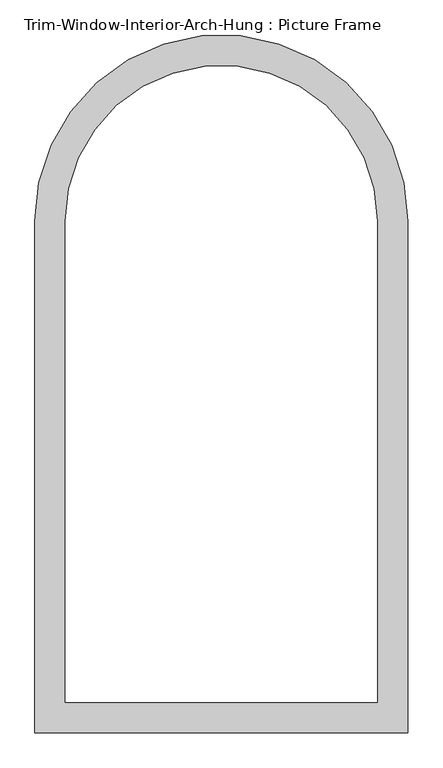
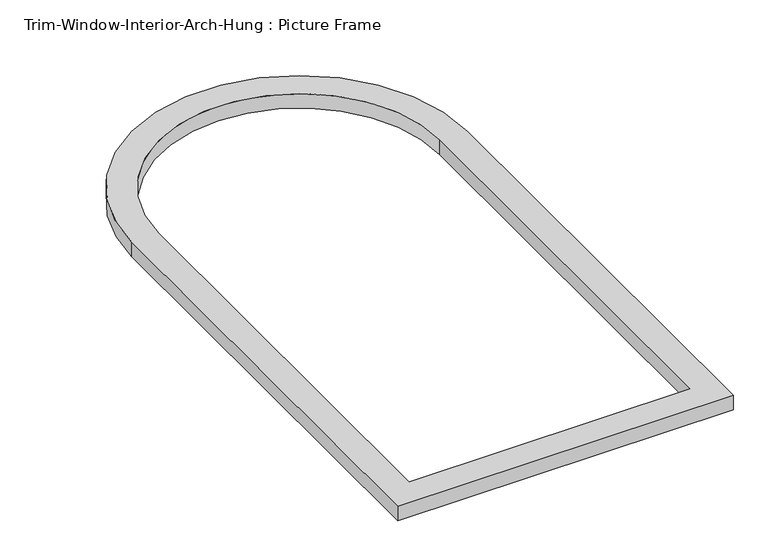
"""IFC4 building model written with IfcOpenShell, lengths in millimetres: proxy geometry, Trim-Window-Interior-Arch-Hung : Picture Frame."""

from ifc_helpers import new_model, si_unit, point, frame_2d, origin, origin_with_axes, place, context, project, spatial, polyline, circle_curve, trimmed, segment, composite_curve, outline, extrude, source, transform, mapped, element, save


def trim_window_interior_arch_hung_picture_frame_76300bdb(model_context):
    return source(origin(), model_context, "Body", "SweptSolid", [
        extrude(outline(composite_curve([segment(trimmed(circle_curve(frame_2d((0.0, -304.8)), 349.25), [point((-349.25, -304.8))], [point((349.25, -304.8))], False, "CARTESIAN"), True, "CONTINUOUS"), segment(polyline([(349.25, -304.8), (349.25, -1263.65), (-349.25, -1263.65), (-349.25, -304.8)]), True, "CONTINUOUS")], self_intersect=False), holes=[composite_curve([segment(polyline([(-292.1, -304.8), (-292.1, -1206.5), (292.1, -1206.5), (292.1, -304.8)]), True, "CONTINUOUS"), segment(trimmed(circle_curve(frame_2d((0.0, -304.8)), 292.1), [point((292.1, -304.8))], [point((-292.1, -304.8))], True, "CARTESIAN"), True, "CONTINUOUS")], self_intersect=False)]), origin_with_axes(), (0.0, 0.0, 1.0), 31.75),
    ])


if __name__ == "__main__":
    model = new_model("IFC4")
    model_context = context("Model", 3, world=origin())
    ifc_project = project(units=[si_unit("LENGTHUNIT", "METRE", prefix="MILLI")], contexts=[model_context])
    site = spatial("IfcSite", under=ifc_project)
    building = spatial("IfcBuilding", under=site)
    placement = place(None, origin())
    trim_window_interior_arch_hung_picture_frame_shape = trim_window_interior_arch_hung_picture_frame_76300bdb(model_context)
    element("IfcBuildingElementProxy", 1, Name="Trim-Window-Interior-Arch-Hung : Picture Frame", ObjectType="Trim-Window-Interior-Arch-Hung : Picture Frame", at=placement, inside=building, context=model_context, shape_type="MappedRepresentation", body=[
        mapped(trim_window_interior_arch_hung_picture_frame_shape, transform((0.0, 0.0, 0.0), x_axis=(1.0, 0.0, 0.0), y_axis=(0.0, 1.0, 0.0), z_axis=(0.0, 0.0, 1.0))),
    ])
    save(model, "model.ifc")

# Revit data of these elements
# Type "Trim-Window-Interior-Arch-Hung : Picture Frame"
#   Trim Thickness_Picture Frame = 0' - 1 1/4"
#   Trim Width = 0' - 2 1/4"
#   Trim Thickness_with Sill = 0' - 0 3/4"
#   Sill Thickness = 0' - 1 1/4"
#   Opening Width [instance default] = 2' - 0"
#   Opening Height [instance default] = 4' - 0"
#   Half Width [instance default] = 1' - 0"
#   Default Elevation = 4' - 0"
#   Sill = no
#   Picture Frame = yes
#   Trim Material [instance default] = none
# Element 1 (IfcBuildingElementProxy, "Trim-Window-Interior-Arch-Hung : Picture Frame")
#   Trim Material = Wood - Stained
#   Materials on its faces: "Wood - Stained"
# Materials
#   "Wood - Stained": class "Wood", colour RGB 224 178 126, transparency 0, Cost = 0
